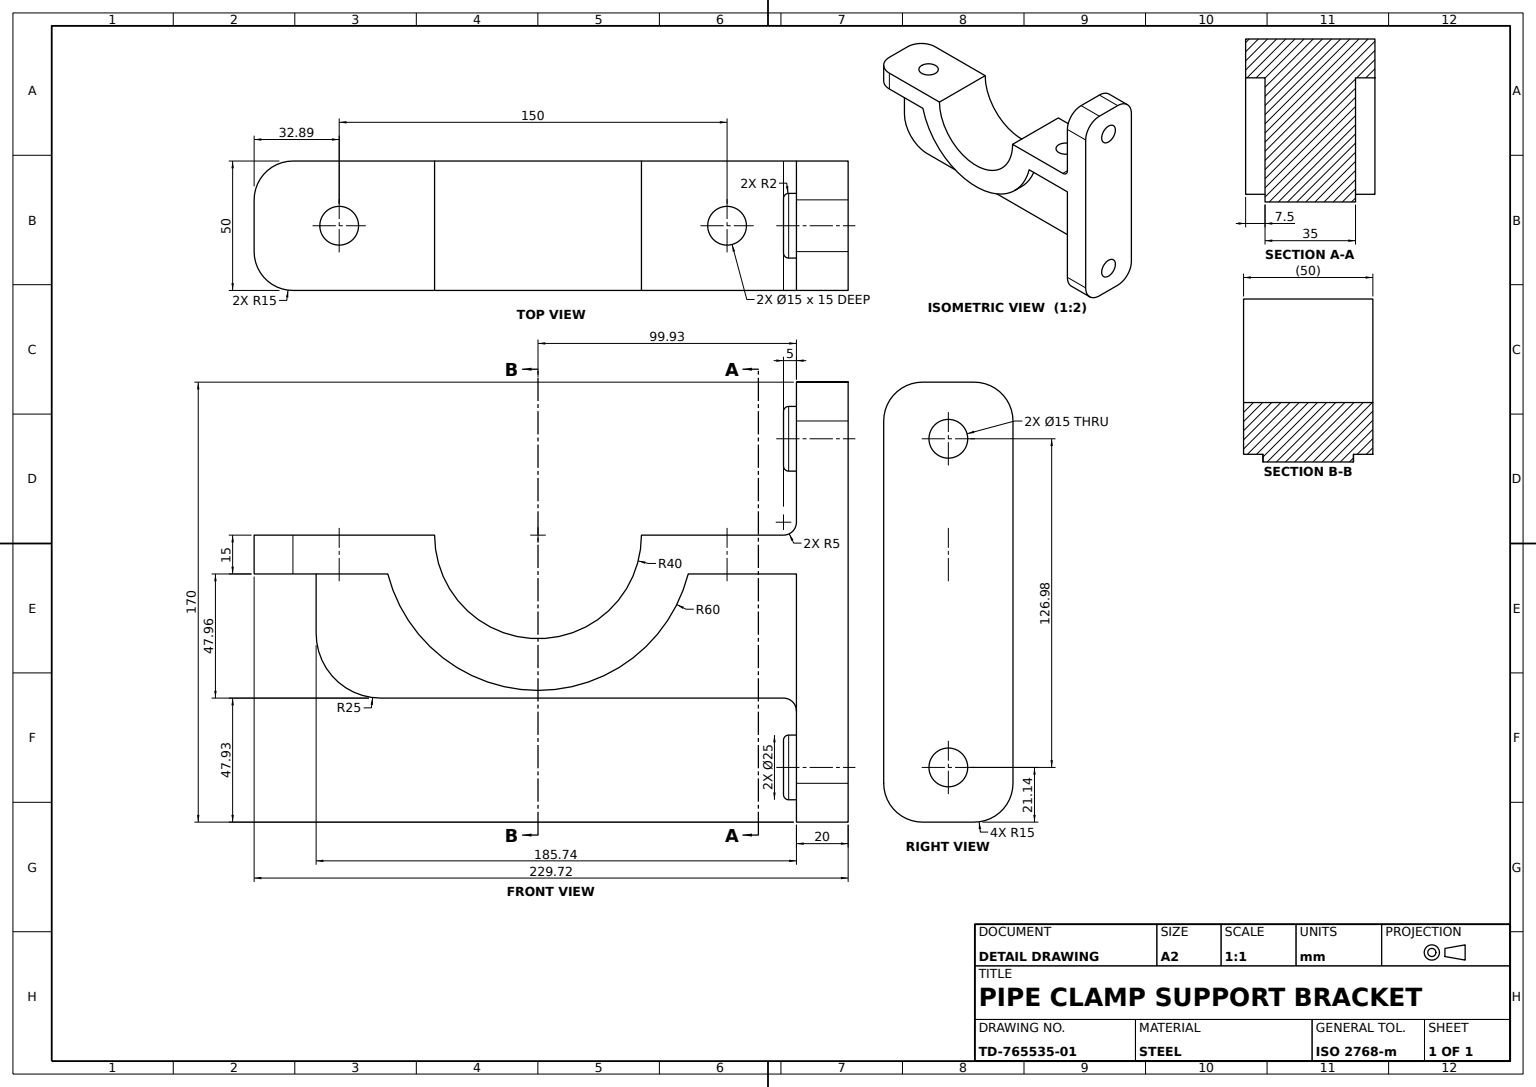
from build123d import *

# Parameters (mm, degrees)
BASE_PLATE_SKETCH_W             = 50
BASE_PLATE_SKETCH_H             = 170
BASE_PLATE_170X50X20_DEPTH      = 20
CLAMP_SADDLE_DEPTH              = 25
SADDLE_FILLET_R15_R             = 15
SADDLE_TO_PLATE_FILLET_R5_R     = 5
CLAMP_BOLT_HOLES_SKETCH_R       = 7.5
CLAMP_BOLT_HOLES_2X_15_DEPTH    = 25
MOUNTING_HOLES_SKETCH_R         = 7.5
MOUNTING_HOLES_2X_15_DEPTH      = 25
MOUNTING_START                  = 5
MOUNTING_HOLE_BOSSES_SKETCH_R   = 12.5
MOUNTING_HOLE_BOSSES_SKETCH_R_2 = 7.5
MOUNTING_HOLE_BOSSES_25_DEPTH   = 5
HOLE_BOSS_FILLET_R2_R           = 2
BASE_PLATE_CORNER_FILLETS_R15_R = 15
SUPPORT_RIB_DEPTH               = 17.5
SUPPORT_RIB_FILLET_R25_R        = 25
RIB_TO_PLATE_FILLET_R5_R        = 5


with BuildPart() as part:
    # Base Plate Sketch → Base Plate 170x50x20 (new body)
    with BuildSketch(Plane.XY):
        Rectangle(BASE_PLATE_SKETCH_W, BASE_PLATE_SKETCH_H)
    extrude(amount=BASE_PLATE_170X50X20_DEPTH)

    # Clamp Saddle Sketch → Clamp Saddle (add, symmetric)
    with BuildSketch(Plane(origin=(0, 0, 0), x_dir=(0, 0, -1), z_dir=(1, 0, 0))):
        with BuildLine():
            Line((-159.934479129, 25.889967638), (-179.934479129, 25.889967638))
            Line((-179.934479129, 25.889967638), (-229.717625742, 25.889967638))
            Line((-229.717625742, 25.889967638), (-229.717625742, 10.889967638))
            Line((-229.717625742, 10.889967638), (-178.029229322, 10.889967638))
            ThreePointArc((-178.029229322, 10.889967638), (-119.934479129, -34.110032362), (-61.839728936, 10.889967638))
            Line((-61.839728936, 10.889967638), (-20, 10.889967638))
            Line((-20, 10.889967638), (-20, 25.889967638))
            Line((-20, 25.889967638), (-79.934479129, 25.889967638))
            ThreePointArc((-79.934479129, 25.889967638), (-119.934479129, -14.110032362), (-159.934479129, 25.889967638))
        make_face()
    extrude(amount=CLAMP_SADDLE_DEPTH, both=True)

    # Saddle Fillet R15
    saddle_fillet_r15_edges = [part.edges().sort_by_distance(p)[0] for p in [
        (25, 18.389967638, 229.717625742),
        (-25, 18.389967638, 229.717625742),
    ]]
    fillet(saddle_fillet_r15_edges, radius=SADDLE_FILLET_R15_R)

    # Saddle To Plate Fillet R5
    saddle_to_plate_fillet_r5_edges = [part.edges().sort_by_distance(p)[0] for p in [
        (0, 25.889967638, 20),
    ]]
    fillet(saddle_to_plate_fillet_r5_edges, radius=SADDLE_TO_PLATE_FILLET_R5_R)

    # Clamp Bolt Holes Sketch → Clamp Bolt Holes 2xØ15 (cut, symmetric)
    with BuildSketch(Plane(origin=(0, 25.889967638, 0), x_dir=(1, 0, 0), z_dir=(0, 1, 0))):
        with Locations(Location((0, -46.822731441, 0), (0, 0, 270))):
            Circle(CLAMP_BOLT_HOLES_SKETCH_R)
        with Locations(Location((0, -196.822731441, 0), (0, 0, 90))):
            Circle(CLAMP_BOLT_HOLES_SKETCH_R)
    extrude(amount=CLAMP_BOLT_HOLES_2X_15_DEPTH, both=True, mode=Mode.SUBTRACT)

    # Mounting Holes Sketch → Mounting Holes 2xØ15 (cut, symmetric)
    with BuildSketch(Plane.XY.offset(20)):
        with Locations((0, 63.122206812)):
            Circle(MOUNTING_HOLES_SKETCH_R)
        with Locations((0, -63.861920173)):
            Circle(MOUNTING_HOLES_SKETCH_R)
    extrude(amount=MOUNTING_HOLES_2X_15_DEPTH, both=True, mode=Mode.SUBTRACT)

    # Mounting Hole Bosses Sketch → Mounting Hole Bosses Ø25 (add)
    # profile 1 of 2: a face of its own
    with BuildSketch(Plane.XY.offset(20).offset(MOUNTING_START)):
        with Locations((0, 63.122206812)):
            Circle(MOUNTING_HOLE_BOSSES_SKETCH_R)
        with Locations((0, 63.122206812)):
            Circle(MOUNTING_HOLE_BOSSES_SKETCH_R_2, mode=Mode.SUBTRACT)
    # profile 2 of 2: a face of its own
    with BuildSketch(Plane.XY.offset(20).offset(MOUNTING_START)):
        with Locations((0, -63.861920173)):
            Circle(MOUNTING_HOLE_BOSSES_SKETCH_R)
        with Locations((0, -63.861920173)):
            Circle(MOUNTING_HOLE_BOSSES_SKETCH_R_2, mode=Mode.SUBTRACT)
    extrude(amount=-MOUNTING_HOLE_BOSSES_25_DEPTH)

    # Hole Boss Fillet R2
    hole_boss_fillet_r2_edges = [part.edges().sort_by_distance(p)[0] for p in [
        (-12.5, 63.122206812, 25),
        (-12.5, -63.861920173, 25),
    ]]
    fillet(hole_boss_fillet_r2_edges, radius=HOLE_BOSS_FILLET_R2_R)

    # Base Plate Corner Fillets R15
    base_plate_corner_fillets_r15_edges = [part.edges().sort_by_distance(p)[0] for p in [
        (25, -85, 10),
        (-25, -85, 10),
        (-25, 85, 10),
        (25, 85, 10),
    ]]
    fillet(base_plate_corner_fillets_r15_edges, radius=BASE_PLATE_CORNER_FILLETS_R15_R)

    # Support Rib Sketch → Support Rib (add, symmetric)
    with BuildSketch(Plane(origin=(0, 0, 0), x_dir=(0, 0, -1), z_dir=(1, 0, 0))):
        with BuildLine():
            Line((-205.743047043, 10.889967638), (-205.743047043, -37.074588444))
            Line((-205.743047043, -37.074588444), (-20, -37.074588444))
            Line((-20, -37.074588444), (-20, 10.889967638))
            Line((-20, 10.889967638), (-61.839728936, 10.889967638))
            ThreePointArc((-61.839728936, 10.889967638), (-119.934479129, -34.110032362), (-178.029229322, 10.889967638))
            Line((-178.029229322, 10.889967638), (-205.743047043, 10.889967638))
        make_face()
    extrude(amount=SUPPORT_RIB_DEPTH, both=True)

    # Support Rib Fillet R25
    support_rib_fillet_r25_edges = [part.edges().sort_by_distance(p)[0] for p in [
        (0, -37.074588444, 205.743047043),
    ]]
    fillet(support_rib_fillet_r25_edges, radius=SUPPORT_RIB_FILLET_R25_R)

    # Rib To Plate Fillet R5
    rib_to_plate_fillet_r5_edges = [part.edges().sort_by_distance(p)[0] for p in [
        (0, -37.074588444, 20),
    ]]
    fillet(rib_to_plate_fillet_r5_edges, radius=RIB_TO_PLATE_FILLET_R5_R)


solid = part.part
